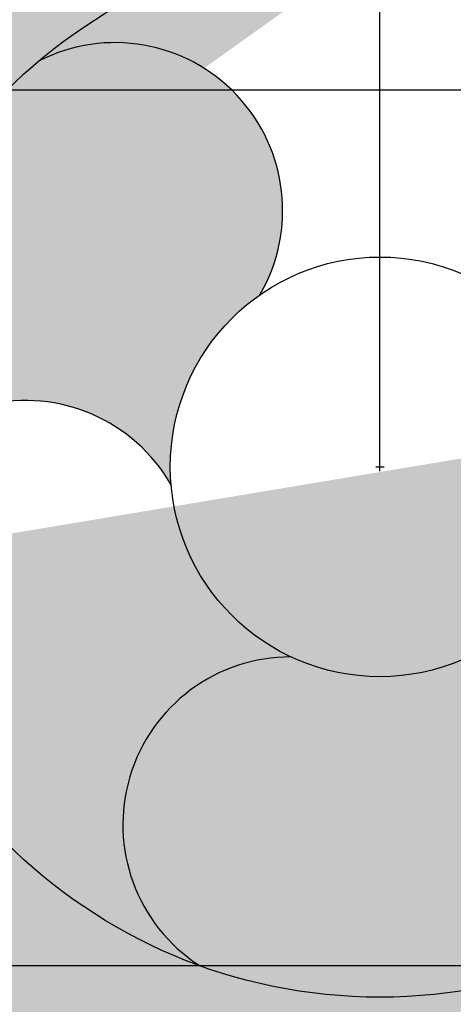
# Model space of a CAD drawing. Units: millimetres. Extents: x -22994 to 29398, y -19990 to 20176.
# Tile 116 of 135: x 220 to 229, y 135 to 156. Entities that reach past the tile are written whole.
import ezdxf

# ---------------------------------------------------------------- set-up
doc = ezdxf.new("R2010")
doc.units = ezdxf.units.MM
doc.header["$MEASUREMENT"] = 0
for name, color, linetype, lineweight in [('M-DIMS', 2, 'Continuous', 18), ('M-EQPM', 7, 'Continuous', 25), ('M-EQPM-PATT', 7, 'Continuous', 18)]:
    doc.layers.add(name, color=color, linetype=linetype, lineweight=lineweight)
doc.styles.get("Standard").update_dxf_attribs({"font": 'arial.ttf'})
doc.dimstyles.get("Standard").update_dxf_attribs({"dimtxt": 0.18, "dimasz": 10000, "dimexe": 0.18, "dimexo": 0.0625, "dimgap": 0.09, "dimtad": 0, "dimtih": 1, "dimtoh": 1, "dimdec": 0, "dimzin": 0, "dimdsep": 46, "dimtxsty": 'Standard', "dimcen": 0.09, "dimadec": 0, "dimazin": 0, "dimtfac": 1, "dimtdec": 0, "dimtofl": 0, "dimtmove": 0, "dimatfit": 3, "dimfxl": 1, "dimtolj": 1, "dimtzin": 0, "dimlwd": 30, "dimarcsym": 0})

# ---------------------------------------------------------------- blocks, each defined once
blk = doc.blocks.new('*D2')
at = {"layer": 'Defpoints', "color": 0, "transparency": 16777216}
for p in [(6.677, 10.271), (290.852, 10.271), (290.852, -5.079)]:
    blk.add_point(p, dxfattribs=at)
at = {"layer": 'M-DIMS', "color": 0, "lineweight": -2, "transparency": 16777216}
for p, q in [((6.677, 10.209), (6.677, -5.259)), ((290.852, 10.209), (290.852, -5.259))]:
    blk.add_line(p, q, dxfattribs=at)
at = {"layer": 'M-DIMS', "color": 0, "lineweight": 30, "transparency": 16777216}
for p, q in [((-9993.323, -5.079), (-19993.323, -5.079)), ((10290.852, -5.079), (20290.852, -5.079))]:
    blk.add_line(p, q, dxfattribs=at)
at = {"layer": 'M-DIMS', "color": 0, "transparency": 16777216}
for points in [[(-9993.323, 1661.588), (-9993.323, -1671.745), (6.677, -5.079)], [(10290.852, 1661.588), (10290.852, -1671.745), (290.852, -5.079)]]:
    blk.add_solid(points, dxfattribs=at)
at = {"layer": 'M-DIMS', "color": 0, "transparency": 16777216, "insert": (148.765, -5.079), "char_height": 0.18, "attachment_point": 5}
blk.add_mtext('\\A1;284.2', dxfattribs=at)
blk = doc.blocks.new('*D3')
at = {"layer": 'Defpoints', "color": 0, "transparency": 16777216}
for p in [(110.265, 204.165), (110.265, 176.366), (95.833, 127.967)]:
    blk.add_point(p, dxfattribs=at)
at = {"layer": 'M-DIMS', "color": 0, "lineweight": -2, "transparency": 16777216}
for p, q in [((95.833, 128.03), (95.833, 204.345)), ((110.265, 176.429), (110.265, 204.345))]:
    blk.add_line(p, q, dxfattribs=at)
at = {"layer": 'M-DIMS', "color": 0, "lineweight": 30, "transparency": 16777216}
for p, q in [((-9904.167, 204.165), (-19904.167, 204.165)), ((10110.265, 204.165), (20110.265, 204.165))]:
    blk.add_line(p, q, dxfattribs=at)
at = {"layer": 'M-DIMS', "color": 0, "transparency": 16777216}
for points in [[(-9904.167, 1870.832), (-9904.167, -1462.501), (95.833, 204.165)], [(10110.265, 1870.832), (10110.265, -1462.501), (110.265, 204.165)]]:
    blk.add_solid(points, dxfattribs=at)
at = {"layer": 'M-DIMS', "color": 0, "transparency": 16777216, "insert": (103.049, 204.165), "char_height": 0.18, "attachment_point": 5}
blk.add_mtext('\\A1;14.432', dxfattribs=at)
blk = doc.blocks.new('*D4')
at = {"layer": 'Defpoints', "color": 0, "transparency": 16777216}
for p in [(116.265, 204.165), (110.265, 176.366), (116.265, 176.366)]:
    blk.add_point(p, dxfattribs=at)
at = {"layer": 'M-DIMS', "color": 0, "lineweight": -2, "transparency": 16777216}
for p, q in [((110.265, 176.429), (110.265, 204.345)), ((116.265, 176.429), (116.265, 204.345))]:
    blk.add_line(p, q, dxfattribs=at)
at = {"layer": 'M-DIMS', "color": 0, "lineweight": 30, "transparency": 16777216}
for p, q in [((-9889.735, 204.165), (-19889.735, 204.165)), ((10116.265, 204.165), (20116.265, 204.165))]:
    blk.add_line(p, q, dxfattribs=at)
at = {"layer": 'M-DIMS', "color": 0, "transparency": 16777216}
for points in [[(-9889.735, 1870.832), (-9889.735, -1462.501), (110.265, 204.165)], [(10116.265, 1870.832), (10116.265, -1462.501), (116.265, 204.165)]]:
    blk.add_solid(points, dxfattribs=at)
at = {"layer": 'M-DIMS', "color": 0, "transparency": 16777216, "insert": (113.265, 204.165), "char_height": 0.18, "attachment_point": 5}
blk.add_mtext('\\A1;6', dxfattribs=at)
blk = doc.blocks.new('*D5')
at = {"layer": 'Defpoints', "color": 0, "transparency": 16777216}
for p in [(181.265, 204.165), (116.265, 176.366), (181.265, 176.366)]:
    blk.add_point(p, dxfattribs=at)
at = {"layer": 'M-DIMS', "color": 0, "lineweight": -2, "transparency": 16777216}
for p, q in [((116.265, 176.429), (116.265, 204.345)), ((181.265, 176.429), (181.265, 204.345))]:
    blk.add_line(p, q, dxfattribs=at)
at = {"layer": 'M-DIMS', "color": 0, "lineweight": 30, "transparency": 16777216}
for p, q in [((-9883.735, 204.165), (-19883.735, 204.165)), ((10181.265, 204.165), (20181.265, 204.165))]:
    blk.add_line(p, q, dxfattribs=at)
at = {"layer": 'M-DIMS', "color": 0, "transparency": 16777216}
for points in [[(-9883.735, 1870.832), (-9883.735, -1462.501), (116.265, 204.165)], [(10181.265, 1870.832), (10181.265, -1462.501), (181.265, 204.165)]]:
    blk.add_solid(points, dxfattribs=at)
at = {"layer": 'M-DIMS', "color": 0, "transparency": 16777216, "insert": (148.765, 204.165), "char_height": 0.18, "attachment_point": 5}
blk.add_mtext('\\A1;65', dxfattribs=at)
blk = doc.blocks.new('*D6')
at = {"layer": 'Defpoints', "color": 0, "transparency": 16777216}
for p in [(187.265, 204.165), (181.265, 176.366), (187.265, 176.366)]:
    blk.add_point(p, dxfattribs=at)
at = {"layer": 'M-DIMS', "color": 0, "lineweight": -2, "transparency": 16777216}
for p, q in [((181.265, 176.429), (181.265, 204.345)), ((187.265, 176.429), (187.265, 204.345))]:
    blk.add_line(p, q, dxfattribs=at)
at = {"layer": 'M-DIMS', "color": 0, "lineweight": 30, "transparency": 16777216}
for p, q in [((-9818.735, 204.165), (-19818.735, 204.165)), ((10187.265, 204.165), (20187.265, 204.165))]:
    blk.add_line(p, q, dxfattribs=at)
at = {"layer": 'M-DIMS', "color": 0, "transparency": 16777216}
for points in [[(-9818.735, 1870.832), (-9818.735, -1462.501), (181.265, 204.165)], [(10187.265, 1870.832), (10187.265, -1462.501), (187.265, 204.165)]]:
    blk.add_solid(points, dxfattribs=at)
at = {"layer": 'M-DIMS', "color": 0, "transparency": 16777216, "insert": (184.265, 204.165), "char_height": 0.18, "attachment_point": 5}
blk.add_mtext('\\A1;6', dxfattribs=at)
blk = doc.blocks.new('*D7')
at = {"layer": 'Defpoints', "color": 0, "transparency": 16777216}
for p in [(201.697, 204.165), (187.265, 176.366), (201.697, 127.967)]:
    blk.add_point(p, dxfattribs=at)
at = {"layer": 'M-DIMS', "color": 0, "lineweight": -2, "transparency": 16777216}
for p, q in [((187.265, 176.429), (187.265, 204.345)), ((201.697, 128.03), (201.697, 204.345))]:
    blk.add_line(p, q, dxfattribs=at)
at = {"layer": 'M-DIMS', "color": 0, "lineweight": 30, "transparency": 16777216}
for p, q in [((-9812.735, 204.165), (-19812.735, 204.165)), ((10201.697, 204.165), (20201.697, 204.165))]:
    blk.add_line(p, q, dxfattribs=at)
at = {"layer": 'M-DIMS', "color": 0, "transparency": 16777216}
for points in [[(-9812.735, 1870.832), (-9812.735, -1462.501), (187.265, 204.165)], [(10201.697, 1870.832), (10201.697, -1462.501), (201.697, 204.165)]]:
    blk.add_solid(points, dxfattribs=at)
at = {"layer": 'M-DIMS', "color": 0, "transparency": 16777216, "insert": (194.481, 204.165), "char_height": 0.18, "attachment_point": 5}
blk.add_mtext('\\A1;14.432', dxfattribs=at)
blk = doc.blocks.new('*D8')
at = {"layer": 'Defpoints', "color": 0, "transparency": 16777216}
for p in [(227.648, 204.165), (227.648, 146.73), (201.697, 127.967)]:
    blk.add_point(p, dxfattribs=at)
at = {"layer": 'M-DIMS', "color": 0, "lineweight": -2, "transparency": 16777216}
for p, q in [((201.697, 128.03), (201.697, 204.345)), ((227.648, 146.792), (227.648, 204.345))]:
    blk.add_line(p, q, dxfattribs=at)
at = {"layer": 'M-DIMS', "color": 0, "lineweight": 30, "transparency": 16777216}
for p, q in [((-9798.303, 204.165), (-19798.303, 204.165)), ((10227.648, 204.165), (20227.648, 204.165))]:
    blk.add_line(p, q, dxfattribs=at)
at = {"layer": 'M-DIMS', "color": 0, "transparency": 16777216}
for points in [[(-9798.303, 1870.832), (-9798.303, -1462.501), (201.697, 204.165)], [(10227.648, 1870.832), (10227.648, -1462.501), (227.648, 204.165)]]:
    blk.add_solid(points, dxfattribs=at)
at = {"layer": 'M-DIMS', "color": 0, "transparency": 16777216, "insert": (214.673, 204.165), "char_height": 0.18, "attachment_point": 5}
blk.add_mtext('\\A1;25.95', dxfattribs=at)
blk = doc.blocks.new('*D9')
at = {"layer": 'Defpoints', "color": 0, "transparency": 16777216}
for p in [(187.265, 176.366), (306.202, 176.366), (290.852, 10.271)]:
    blk.add_point(p, dxfattribs=at)
at = {"layer": 'M-DIMS', "color": 0, "lineweight": 30, "transparency": 16777216}
for p, q in [((306.202, 10176.366), (306.202, 20176.366)), ((306.202, -9989.729), (306.202, -19989.729))]:
    blk.add_line(p, q, dxfattribs=at)
at = {"layer": 'M-DIMS', "color": 0, "lineweight": -2, "transparency": 16777216}
for p, q in [((187.327, 176.366), (306.382, 176.366)), ((290.915, 10.271), (306.382, 10.271))]:
    blk.add_line(p, q, dxfattribs=at)
at = {"layer": 'M-DIMS', "color": 0, "transparency": 16777216}
for points in [[(-1360.465, 10176.366), (1972.869, 10176.366), (306.202, 176.366)], [(-1360.465, -9989.729), (1972.869, -9989.729), (306.202, 10.271)]]:
    blk.add_solid(points, dxfattribs=at)
at = {"layer": 'M-DIMS', "color": 0, "transparency": 16777216, "insert": (306.202, 93.319), "char_height": 0.18, "attachment_point": 5}
blk.add_mtext('\\A1;166.1', dxfattribs=at)
blk = doc.blocks.new('*D10')
at = {"layer": 'Defpoints', "color": 0, "transparency": 16777216}
for p in [(125.65, 136.071), (133.346, 136.071), (133.346, -5.079)]:
    blk.add_point(p, dxfattribs=at)
at = {"layer": 'M-DIMS', "color": 0, "lineweight": -2, "transparency": 16777216}
for p, q in [((125.65, 136.009), (125.65, -5.259)), ((133.346, 136.009), (133.346, -5.259))]:
    blk.add_line(p, q, dxfattribs=at)
at = {"layer": 'M-DIMS', "color": 0, "lineweight": 30, "transparency": 16777216}
for p, q in [((-9874.35, -5.079), (-19874.35, -5.079)), ((10133.346, -5.079), (20133.346, -5.079))]:
    blk.add_line(p, q, dxfattribs=at)
at = {"layer": 'M-DIMS', "color": 0, "transparency": 16777216}
for points in [[(-9874.35, 1661.588), (-9874.35, -1671.745), (125.65, -5.079)], [(10133.346, 1661.588), (10133.346, -1671.745), (133.346, -5.079)]]:
    blk.add_solid(points, dxfattribs=at)
at = {"layer": 'M-DIMS', "color": 0, "transparency": 16777216, "insert": (129.498, -5.079), "char_height": 0.18, "attachment_point": 5}
blk.add_mtext('\\A1;7.696', dxfattribs=at)
blk = doc.blocks.new('*D11')
at = {"layer": 'Defpoints', "color": 0, "transparency": 16777216}
for p in [(133.346, 136.071), (135.65, 136.071), (135.65, -5.079)]:
    blk.add_point(p, dxfattribs=at)
at = {"layer": 'M-DIMS', "color": 0, "lineweight": -2, "transparency": 16777216}
for p, q in [((133.346, 136.009), (133.346, -5.259)), ((135.65, 136.009), (135.65, -5.259))]:
    blk.add_line(p, q, dxfattribs=at)
at = {"layer": 'M-DIMS', "color": 0, "lineweight": 30, "transparency": 16777216}
for p, q in [((-9866.654, -5.079), (-19866.654, -5.079)), ((10135.65, -5.079), (20135.65, -5.079))]:
    blk.add_line(p, q, dxfattribs=at)
at = {"layer": 'M-DIMS', "color": 0, "transparency": 16777216}
for points in [[(-9866.654, 1661.588), (-9866.654, -1671.745), (133.346, -5.079)], [(10135.65, 1661.588), (10135.65, -1671.745), (135.65, -5.079)]]:
    blk.add_solid(points, dxfattribs=at)
at = {"layer": 'M-DIMS', "color": 0, "transparency": 16777216, "insert": (134.498, -5.079), "char_height": 0.18, "attachment_point": 5}
blk.add_mtext('\\A1;2.304', dxfattribs=at)
blk = doc.blocks.new('*D12')
at = {"layer": 'Defpoints', "color": 0, "transparency": 16777216}
for p in [(135.65, 136.071), (145.65, 136.071), (145.65, -5.079)]:
    blk.add_point(p, dxfattribs=at)
at = {"layer": 'M-DIMS', "color": 0, "lineweight": -2, "transparency": 16777216}
for p, q in [((135.65, 136.009), (135.65, -5.259)), ((145.65, 136.009), (145.65, -5.259))]:
    blk.add_line(p, q, dxfattribs=at)
at = {"layer": 'M-DIMS', "color": 0, "lineweight": 30, "transparency": 16777216}
for p, q in [((-9864.35, -5.079), (-19864.35, -5.079)), ((10145.65, -5.079), (20145.65, -5.079))]:
    blk.add_line(p, q, dxfattribs=at)
at = {"layer": 'M-DIMS', "color": 0, "transparency": 16777216}
for points in [[(-9864.35, 1661.588), (-9864.35, -1671.745), (135.65, -5.079)], [(10145.65, 1661.588), (10145.65, -1671.745), (145.65, -5.079)]]:
    blk.add_solid(points, dxfattribs=at)
at = {"layer": 'M-DIMS', "color": 0, "transparency": 16777216, "insert": (140.65, -5.079), "char_height": 0.18, "attachment_point": 5}
blk.add_mtext('\\A1;10', dxfattribs=at)
blk = doc.blocks.new('*D13')
at = {"layer": 'Defpoints', "color": 0, "transparency": 16777216}
for p in [(145.65, 136.071), (155.65, 136.071), (155.65, -5.079)]:
    blk.add_point(p, dxfattribs=at)
at = {"layer": 'M-DIMS', "color": 0, "lineweight": -2, "transparency": 16777216}
for p, q in [((145.65, 136.009), (145.65, -5.259)), ((155.65, 136.009), (155.65, -5.259))]:
    blk.add_line(p, q, dxfattribs=at)
at = {"layer": 'M-DIMS', "color": 0, "lineweight": 30, "transparency": 16777216}
for p, q in [((-9854.35, -5.079), (-19854.35, -5.079)), ((10155.65, -5.079), (20155.65, -5.079))]:
    blk.add_line(p, q, dxfattribs=at)
at = {"layer": 'M-DIMS', "color": 0, "transparency": 16777216}
for points in [[(-9854.35, 1661.588), (-9854.35, -1671.745), (145.65, -5.079)], [(10155.65, 1661.588), (10155.65, -1671.745), (155.65, -5.079)]]:
    blk.add_solid(points, dxfattribs=at)
at = {"layer": 'M-DIMS', "color": 0, "transparency": 16777216, "insert": (150.65, -5.079), "char_height": 0.18, "attachment_point": 5}
blk.add_mtext('\\A1;10', dxfattribs=at)
blk = doc.blocks.new('*D14')
at = {"layer": 'Defpoints', "color": 0, "transparency": 16777216}
for p in [(155.65, 136.071), (165.65, 136.071), (165.65, -5.079)]:
    blk.add_point(p, dxfattribs=at)
at = {"layer": 'M-DIMS', "color": 0, "lineweight": -2, "transparency": 16777216}
for p, q in [((155.65, 136.009), (155.65, -5.259)), ((165.65, 136.009), (165.65, -5.259))]:
    blk.add_line(p, q, dxfattribs=at)
at = {"layer": 'M-DIMS', "color": 0, "lineweight": 30, "transparency": 16777216}
for p, q in [((-9844.35, -5.079), (-19844.35, -5.079)), ((10165.65, -5.079), (20165.65, -5.079))]:
    blk.add_line(p, q, dxfattribs=at)
at = {"layer": 'M-DIMS', "color": 0, "transparency": 16777216}
for points in [[(-9844.35, 1661.588), (-9844.35, -1671.745), (155.65, -5.079)], [(10165.65, 1661.588), (10165.65, -1671.745), (165.65, -5.079)]]:
    blk.add_solid(points, dxfattribs=at)
at = {"layer": 'M-DIMS', "color": 0, "transparency": 16777216, "insert": (160.65, -5.079), "char_height": 0.18, "attachment_point": 5}
blk.add_mtext('\\A1;10', dxfattribs=at)
blk = doc.blocks.new('*D15')
at = {"layer": 'Defpoints', "color": 0, "transparency": 16777216}
for p in [(173.346, 154.788), (173.346, 136.071), (306.202, 136.071)]:
    blk.add_point(p, dxfattribs=at)
at = {"layer": 'M-DIMS', "color": 0, "lineweight": 30, "transparency": 16777216}
for p, q in [((306.202, 10154.788), (306.202, 20154.788)), ((306.202, -9863.929), (306.202, -19863.929))]:
    blk.add_line(p, q, dxfattribs=at)
at = {"layer": 'M-DIMS', "color": 0, "lineweight": -2, "transparency": 16777216}
for p, q in [((173.408, 154.788), (306.382, 154.788)), ((173.408, 136.071), (306.382, 136.071))]:
    blk.add_line(p, q, dxfattribs=at)
at = {"layer": 'M-DIMS', "color": 0, "transparency": 16777216}
for points in [[(-1360.465, 10154.788), (1972.869, 10154.788), (306.202, 154.788)], [(-1360.465, -9863.929), (1972.869, -9863.929), (306.202, 136.071)]]:
    blk.add_solid(points, dxfattribs=at)
at = {"layer": 'M-DIMS', "color": 0, "transparency": 16777216, "insert": (306.202, 145.43), "char_height": 0.18, "attachment_point": 5}
blk.add_mtext('\\A1;18.717', dxfattribs=at)
blk = doc.blocks.new('*D16')
at = {"layer": 'Defpoints', "color": 0, "transparency": 16777216}
for p in [(120.17, 204.165), (110.466, 48.035), (120.17, 48.035)]:
    blk.add_point(p, dxfattribs=at)
at = {"layer": 'M-DIMS', "color": 0, "lineweight": -2, "transparency": 16777216}
for p, q in [((110.466, 48.097), (110.466, 204.345)), ((120.17, 48.097), (120.17, 204.345))]:
    blk.add_line(p, q, dxfattribs=at)
at = {"layer": 'M-DIMS', "color": 0, "lineweight": 30, "transparency": 16777216}
for p, q in [((-9889.534, 204.165), (-19889.534, 204.165)), ((10120.17, 204.165), (20120.17, 204.165))]:
    blk.add_line(p, q, dxfattribs=at)
at = {"layer": 'M-DIMS', "color": 0, "transparency": 16777216}
for points in [[(-9889.534, 1870.832), (-9889.534, -1462.501), (110.466, 204.165)], [(10120.17, 1870.832), (10120.17, -1462.501), (120.17, 204.165)]]:
    blk.add_solid(points, dxfattribs=at)
at = {"layer": 'M-DIMS', "color": 0, "transparency": 16777216, "insert": (115.318, 204.165), "char_height": 0.18, "attachment_point": 5}
blk.add_mtext('\\A1;9.704', dxfattribs=at)
blk = doc.blocks.new('*D17')
at = {"layer": 'Defpoints', "color": 0, "transparency": 16777216}
for p in [(126.17, 204.165), (120.17, 48.035), (126.17, 48.035)]:
    blk.add_point(p, dxfattribs=at)
at = {"layer": 'M-DIMS', "color": 0, "lineweight": -2, "transparency": 16777216}
for p, q in [((120.17, 48.097), (120.17, 204.345)), ((126.17, 48.097), (126.17, 204.345))]:
    blk.add_line(p, q, dxfattribs=at)
at = {"layer": 'M-DIMS', "color": 0, "lineweight": 30, "transparency": 16777216}
for p, q in [((-9879.83, 204.165), (-19879.83, 204.165)), ((10126.17, 204.165), (20126.17, 204.165))]:
    blk.add_line(p, q, dxfattribs=at)
at = {"layer": 'M-DIMS', "color": 0, "transparency": 16777216}
for points in [[(-9879.83, 1870.832), (-9879.83, -1462.501), (120.17, 204.165)], [(10126.17, 1870.832), (10126.17, -1462.501), (126.17, 204.165)]]:
    blk.add_solid(points, dxfattribs=at)
at = {"layer": 'M-DIMS', "color": 0, "transparency": 16777216, "insert": (123.17, 204.165), "char_height": 0.18, "attachment_point": 5}
blk.add_mtext('\\A1;6', dxfattribs=at)
blk = doc.blocks.new('*D18')
at = {"layer": 'Defpoints', "color": 0, "transparency": 16777216}
for p in [(132.17, 204.165), (126.17, 48.035), (132.17, 48.035)]:
    blk.add_point(p, dxfattribs=at)
at = {"layer": 'M-DIMS', "color": 0, "lineweight": -2, "transparency": 16777216}
for p, q in [((126.17, 48.097), (126.17, 204.345)), ((132.17, 48.097), (132.17, 204.345))]:
    blk.add_line(p, q, dxfattribs=at)
at = {"layer": 'M-DIMS', "color": 0, "lineweight": 30, "transparency": 16777216}
for p, q in [((-9873.83, 204.165), (-19873.83, 204.165)), ((10132.17, 204.165), (20132.17, 204.165))]:
    blk.add_line(p, q, dxfattribs=at)
at = {"layer": 'M-DIMS', "color": 0, "transparency": 16777216}
for points in [[(-9873.83, 1870.832), (-9873.83, -1462.501), (126.17, 204.165)], [(10132.17, 1870.832), (10132.17, -1462.501), (132.17, 204.165)]]:
    blk.add_solid(points, dxfattribs=at)
at = {"layer": 'M-DIMS', "color": 0, "transparency": 16777216, "insert": (129.17, 204.165), "char_height": 0.18, "attachment_point": 5}
blk.add_mtext('\\A1;6', dxfattribs=at)
blk = doc.blocks.new('*D19')
at = {"layer": 'Defpoints', "color": 0, "transparency": 16777216}
for p in [(138.17, 204.165), (132.17, 48.035), (138.17, 48.035)]:
    blk.add_point(p, dxfattribs=at)
at = {"layer": 'M-DIMS', "color": 0, "lineweight": -2, "transparency": 16777216}
for p, q in [((132.17, 48.097), (132.17, 204.345)), ((138.17, 48.097), (138.17, 204.345))]:
    blk.add_line(p, q, dxfattribs=at)
at = {"layer": 'M-DIMS', "color": 0, "lineweight": 30, "transparency": 16777216}
for p, q in [((-9867.83, 204.165), (-19867.83, 204.165)), ((10138.17, 204.165), (20138.17, 204.165))]:
    blk.add_line(p, q, dxfattribs=at)
at = {"layer": 'M-DIMS', "color": 0, "transparency": 16777216}
for points in [[(-9867.83, 1870.832), (-9867.83, -1462.501), (132.17, 204.165)], [(10138.17, 1870.832), (10138.17, -1462.501), (138.17, 204.165)]]:
    blk.add_solid(points, dxfattribs=at)
at = {"layer": 'M-DIMS', "color": 0, "transparency": 16777216, "insert": (135.17, 204.165), "char_height": 0.18, "attachment_point": 5}
blk.add_mtext('\\A1;6', dxfattribs=at)
blk = doc.blocks.new('*D20')
at = {"layer": 'Defpoints', "color": 0, "transparency": 16777216}
for p in [(144.17, 204.165), (138.17, 48.035), (144.17, 48.035)]:
    blk.add_point(p, dxfattribs=at)
at = {"layer": 'M-DIMS', "color": 0, "lineweight": -2, "transparency": 16777216}
for p, q in [((138.17, 48.097), (138.17, 204.345)), ((144.17, 48.097), (144.17, 204.345))]:
    blk.add_line(p, q, dxfattribs=at)
at = {"layer": 'M-DIMS', "color": 0, "lineweight": 30, "transparency": 16777216}
for p, q in [((-9861.83, 204.165), (-19861.83, 204.165)), ((10144.17, 204.165), (20144.17, 204.165))]:
    blk.add_line(p, q, dxfattribs=at)
at = {"layer": 'M-DIMS', "color": 0, "transparency": 16777216}
for points in [[(-9861.83, 1870.832), (-9861.83, -1462.501), (138.17, 204.165)], [(10144.17, 1870.832), (10144.17, -1462.501), (144.17, 204.165)]]:
    blk.add_solid(points, dxfattribs=at)
at = {"layer": 'M-DIMS', "color": 0, "transparency": 16777216, "insert": (141.17, 204.165), "char_height": 0.18, "attachment_point": 5}
blk.add_mtext('\\A1;6', dxfattribs=at)
blk = doc.blocks.new('*D21')
at = {"layer": 'Defpoints', "color": 0, "transparency": 16777216}
for p in [(149.116, 204.165), (144.17, 48.035), (149.116, 48.035)]:
    blk.add_point(p, dxfattribs=at)
at = {"layer": 'M-DIMS', "color": 0, "lineweight": -2, "transparency": 16777216}
for p, q in [((144.17, 48.097), (144.17, 204.345)), ((149.116, 48.097), (149.116, 204.345))]:
    blk.add_line(p, q, dxfattribs=at)
at = {"layer": 'M-DIMS', "color": 0, "lineweight": 30, "transparency": 16777216}
for p, q in [((-9855.83, 204.165), (-19855.83, 204.165)), ((10149.116, 204.165), (20149.116, 204.165))]:
    blk.add_line(p, q, dxfattribs=at)
at = {"layer": 'M-DIMS', "color": 0, "transparency": 16777216}
for points in [[(-9855.83, 1870.832), (-9855.83, -1462.501), (144.17, 204.165)], [(10149.116, 1870.832), (10149.116, -1462.501), (149.116, 204.165)]]:
    blk.add_solid(points, dxfattribs=at)
at = {"layer": 'M-DIMS', "color": 0, "transparency": 16777216, "insert": (146.643, 204.165), "char_height": 0.18, "attachment_point": 5}
blk.add_mtext('\\A1;4.945', dxfattribs=at)
blk = doc.blocks.new('*D22')
at = {"layer": 'Defpoints', "color": 0, "transparency": 16777216}
for p in [(149.116, 30.99), (155.116, 30.99), (155.116, -5.079)]:
    blk.add_point(p, dxfattribs=at)
at = {"layer": 'M-DIMS', "color": 0, "lineweight": -2, "transparency": 16777216}
for p, q in [((149.116, 30.927), (149.116, -5.259)), ((155.116, 30.927), (155.116, -5.259))]:
    blk.add_line(p, q, dxfattribs=at)
at = {"layer": 'M-DIMS', "color": 0, "lineweight": 30, "transparency": 16777216}
for p, q in [((-9850.884, -5.079), (-19850.884, -5.079)), ((10155.116, -5.079), (20155.116, -5.079))]:
    blk.add_line(p, q, dxfattribs=at)
at = {"layer": 'M-DIMS', "color": 0, "transparency": 16777216}
for points in [[(-9850.884, 1661.588), (-9850.884, -1671.745), (149.116, -5.079)], [(10155.116, 1661.588), (10155.116, -1671.745), (155.116, -5.079)]]:
    blk.add_solid(points, dxfattribs=at)
at = {"layer": 'M-DIMS', "color": 0, "transparency": 16777216, "insert": (152.116, -5.079), "char_height": 0.18, "attachment_point": 5}
blk.add_mtext('\\A1;6', dxfattribs=at)
blk = doc.blocks.new('*D23')
at = {"layer": 'Defpoints', "color": 0, "transparency": 16777216}
for p in [(155.116, 30.99), (161.116, 30.99), (161.116, -5.079)]:
    blk.add_point(p, dxfattribs=at)
at = {"layer": 'M-DIMS', "color": 0, "lineweight": -2, "transparency": 16777216}
for p, q in [((155.116, 30.927), (155.116, -5.259)), ((161.116, 30.927), (161.116, -5.259))]:
    blk.add_line(p, q, dxfattribs=at)
at = {"layer": 'M-DIMS', "color": 0, "lineweight": 30, "transparency": 16777216}
for p, q in [((-9844.884, -5.079), (-19844.884, -5.079)), ((10161.116, -5.079), (20161.116, -5.079))]:
    blk.add_line(p, q, dxfattribs=at)
at = {"layer": 'M-DIMS', "color": 0, "transparency": 16777216}
for points in [[(-9844.884, 1661.588), (-9844.884, -1671.745), (155.116, -5.079)], [(10161.116, 1661.588), (10161.116, -1671.745), (161.116, -5.079)]]:
    blk.add_solid(points, dxfattribs=at)
at = {"layer": 'M-DIMS', "color": 0, "transparency": 16777216, "insert": (158.116, -5.079), "char_height": 0.18, "attachment_point": 5}
blk.add_mtext('\\A1;6', dxfattribs=at)
blk = doc.blocks.new('*D24')
at = {"layer": 'Defpoints', "color": 0, "transparency": 16777216}
for p in [(161.116, 30.99), (166.439, 30.99), (166.439, -5.079)]:
    blk.add_point(p, dxfattribs=at)
at = {"layer": 'M-DIMS', "color": 0, "lineweight": -2, "transparency": 16777216}
for p, q in [((161.116, 30.927), (161.116, -5.259)), ((166.439, 30.927), (166.439, -5.259))]:
    blk.add_line(p, q, dxfattribs=at)
at = {"layer": 'M-DIMS', "color": 0, "lineweight": 30, "transparency": 16777216}
for p, q in [((-9838.884, -5.079), (-19838.884, -5.079)), ((10166.439, -5.079), (20166.439, -5.079))]:
    blk.add_line(p, q, dxfattribs=at)
at = {"layer": 'M-DIMS', "color": 0, "transparency": 16777216}
for points in [[(-9838.884, 1661.588), (-9838.884, -1671.745), (161.116, -5.079)], [(10166.439, 1661.588), (10166.439, -1671.745), (166.439, -5.079)]]:
    blk.add_solid(points, dxfattribs=at)
at = {"layer": 'M-DIMS', "color": 0, "transparency": 16777216, "insert": (163.777, -5.079), "char_height": 0.18, "attachment_point": 5}
blk.add_mtext('\\A1;5.323', dxfattribs=at)
blk = doc.blocks.new('*D25')
at = {"layer": 'Defpoints', "color": 0, "transparency": 16777216}
for p in [(166.439, 30.99), (172.439, 30.99), (172.439, -5.079)]:
    blk.add_point(p, dxfattribs=at)
at = {"layer": 'M-DIMS', "color": 0, "lineweight": -2, "transparency": 16777216}
for p, q in [((166.439, 30.927), (166.439, -5.259)), ((172.439, 30.927), (172.439, -5.259))]:
    blk.add_line(p, q, dxfattribs=at)
at = {"layer": 'M-DIMS', "color": 0, "lineweight": 30, "transparency": 16777216}
for p, q in [((-9833.561, -5.079), (-19833.561, -5.079)), ((10172.439, -5.079), (20172.439, -5.079))]:
    blk.add_line(p, q, dxfattribs=at)
at = {"layer": 'M-DIMS', "color": 0, "transparency": 16777216}
for points in [[(-9833.561, 1661.588), (-9833.561, -1671.745), (166.439, -5.079)], [(10172.439, 1661.588), (10172.439, -1671.745), (172.439, -5.079)]]:
    blk.add_solid(points, dxfattribs=at)
at = {"layer": 'M-DIMS', "color": 0, "transparency": 16777216, "insert": (169.439, -5.079), "char_height": 0.18, "attachment_point": 5}
blk.add_mtext('\\A1;6', dxfattribs=at)
blk = doc.blocks.new('*D26')
at = {"layer": 'Defpoints', "color": 0, "transparency": 16777216}
for p in [(172.439, 30.99), (178.439, 30.99), (178.439, -5.079)]:
    blk.add_point(p, dxfattribs=at)
at = {"layer": 'M-DIMS', "color": 0, "lineweight": -2, "transparency": 16777216}
for p, q in [((172.439, 30.927), (172.439, -5.259)), ((178.439, 30.927), (178.439, -5.259))]:
    blk.add_line(p, q, dxfattribs=at)
at = {"layer": 'M-DIMS', "color": 0, "lineweight": 30, "transparency": 16777216}
for p, q in [((-9827.561, -5.079), (-19827.561, -5.079)), ((10178.439, -5.079), (20178.439, -5.079))]:
    blk.add_line(p, q, dxfattribs=at)
at = {"layer": 'M-DIMS', "color": 0, "transparency": 16777216}
for points in [[(-9827.561, 1661.588), (-9827.561, -1671.745), (172.439, -5.079)], [(10178.439, 1661.588), (10178.439, -1671.745), (178.439, -5.079)]]:
    blk.add_solid(points, dxfattribs=at)
at = {"layer": 'M-DIMS', "color": 0, "transparency": 16777216, "insert": (175.439, -5.079), "char_height": 0.18, "attachment_point": 5}
blk.add_mtext('\\A1;6', dxfattribs=at)
blk = doc.blocks.new('*D27')
at = {"layer": 'Defpoints', "color": 0, "transparency": 16777216}
for p in [(178.439, 30.99), (188.117, 30.99), (188.117, -5.079)]:
    blk.add_point(p, dxfattribs=at)
at = {"layer": 'M-DIMS', "color": 0, "lineweight": -2, "transparency": 16777216}
for p, q in [((178.439, 30.927), (178.439, -5.259)), ((188.117, 30.927), (188.117, -5.259))]:
    blk.add_line(p, q, dxfattribs=at)
at = {"layer": 'M-DIMS', "color": 0, "lineweight": 30, "transparency": 16777216}
for p, q in [((-9821.561, -5.079), (-19821.561, -5.079)), ((10188.117, -5.079), (20188.117, -5.079))]:
    blk.add_line(p, q, dxfattribs=at)
at = {"layer": 'M-DIMS', "color": 0, "transparency": 16777216}
for points in [[(-9821.561, 1661.588), (-9821.561, -1671.745), (178.439, -5.079)], [(10188.117, 1661.588), (10188.117, -1671.745), (188.117, -5.079)]]:
    blk.add_solid(points, dxfattribs=at)
at = {"layer": 'M-DIMS', "color": 0, "transparency": 16777216, "insert": (183.278, -5.079), "char_height": 0.18, "attachment_point": 5}
blk.add_mtext('\\A1;9.679', dxfattribs=at)
blk = doc.blocks.new('*D28')
at = {"layer": 'Defpoints', "color": 0, "transparency": 16777216}
for p in [(188.117, 48.035), (306.202, 48.035), (188.117, 30.99)]:
    blk.add_point(p, dxfattribs=at)
at = {"layer": 'M-DIMS', "color": 0, "lineweight": 30, "transparency": 16777216}
for p, q in [((306.202, 10048.035), (306.202, 20048.035)), ((306.202, -9969.01), (306.202, -19969.01))]:
    blk.add_line(p, q, dxfattribs=at)
at = {"layer": 'M-DIMS', "color": 0, "lineweight": -2, "transparency": 16777216}
for p, q in [((188.18, 48.035), (306.382, 48.035)), ((188.18, 30.99), (306.382, 30.99))]:
    blk.add_line(p, q, dxfattribs=at)
at = {"layer": 'M-DIMS', "color": 0, "transparency": 16777216}
for points in [[(-1360.465, 10048.035), (1972.869, 10048.035), (306.202, 48.035)], [(-1360.465, -9969.01), (1972.869, -9969.01), (306.202, 30.99)]]:
    blk.add_solid(points, dxfattribs=at)
at = {"layer": 'M-DIMS', "color": 0, "transparency": 16777216, "insert": (306.202, 39.512), "char_height": 0.18, "attachment_point": 5}
blk.add_mtext('\\A1;17.045', dxfattribs=at)
blk = doc.blocks.new('*D29')
at = {"layer": 'Defpoints', "color": 0, "transparency": 16777216}
for p in [(36.801, 80.045), (64.03, 80.045)]:
    blk.add_point(p, dxfattribs=at)
at = {"layer": 'M-DIMS', "color": 0, "lineweight": -2, "transparency": 16777216}
for p, q in [((50.325, 80.045), (50.505, 80.045)), ((50.415, 79.955), (50.415, 80.135))]:
    blk.add_line(p, q, dxfattribs=at)
at = {"layer": 'M-DIMS', "color": 0, "lineweight": 30, "transparency": 16777216}
blk.add_line((20064.03, 80.03), (10064.03, 80.038), dxfattribs=at)
at = {"layer": 'M-DIMS', "color": 0, "transparency": 16777216}
blk.add_solid([(10064.031, 1746.704), (10064.028, -1586.629), (64.03, 80.045)], dxfattribs=at)
at = {"layer": 'M-DIMS', "color": 0, "transparency": 16777216, "insert": (20064.521, 80.03), "char_height": 0.18, "attachment_point": 5}
blk.add_mtext('\\A1;∅27.23', dxfattribs=at)
blk = doc.blocks.new('*D30')
at = {"layer": 'Defpoints', "color": 0, "transparency": 16777216}
for p in [(216.315, 146.729), (238.982, 146.73)]:
    blk.add_point(p, dxfattribs=at)
at = {"layer": 'M-DIMS', "color": 0, "lineweight": 30, "transparency": 16777216}
blk.add_line((20238.982, 147.496), (10238.982, 147.113), dxfattribs=at)
at = {"layer": 'M-DIMS', "color": 0, "lineweight": -2, "transparency": 16777216}
for p, q in [((227.558, 146.73), (227.738, 146.73)), ((227.648, 146.64), (227.648, 146.82))]:
    blk.add_line(p, q, dxfattribs=at)
at = {"layer": 'M-DIMS', "color": 0, "transparency": 16777216}
blk.add_solid([(10238.918, 1813.78), (10239.046, -1519.554), (238.982, 146.73)], dxfattribs=at)
at = {"layer": 'M-DIMS', "color": 0, "transparency": 16777216, "insert": (20239.544, 147.496), "char_height": 0.18, "attachment_point": 5}
blk.add_mtext('\\A1;∅22.667', dxfattribs=at)
blk = doc.blocks.new('*D31')
at = {"layer": 'Defpoints', "color": 0, "transparency": 16777216}
for p in [(223.164, 146.729), (232.133, 146.73)]:
    blk.add_point(p, dxfattribs=at)
at = {"layer": 'M-DIMS', "color": 0, "lineweight": 30, "transparency": 16777216}
blk.add_line((20232.133, 148.666), (10232.133, 147.698), dxfattribs=at)
at = {"layer": 'M-DIMS', "color": 0, "lineweight": -2, "transparency": 16777216}
for p, q in [((227.558, 146.73), (227.738, 146.73)), ((227.648, 146.64), (227.648, 146.82))]:
    blk.add_line(p, q, dxfattribs=at)
at = {"layer": 'M-DIMS', "color": 0, "transparency": 16777216}
blk.add_solid([(10231.971, 1814.364), (10232.294, -1518.969), (232.133, 146.73)], dxfattribs=at)
at = {"layer": 'M-DIMS', "color": 0, "transparency": 16777216, "insert": (20232.625, 148.666), "char_height": 0.18, "attachment_point": 5}
blk.add_mtext('\\A1;∅8.969', dxfattribs=at)
blk = doc.blocks.new('*D34')
at = {"layer": 'Defpoints', "color": 0, "transparency": 16777216}
for p in [(178.58, 122.895), (176.812, 121.128)]:
    blk.add_point(p, dxfattribs=at)
at = {"layer": 'M-DIMS', "color": 0, "lineweight": 30, "transparency": 16777216}
for p, q in [((14322.436, 14263.311), (7250.508, 7193.103)), ((24322.436, 14263.311), (14322.436, 14263.311))]:
    blk.add_line(p, q, dxfattribs=at)
at = {"layer": 'M-DIMS', "color": 0, "lineweight": -2, "transparency": 16777216}
for p, q in [((176.812, 121.038), (176.812, 121.218)), ((176.722, 121.128), (176.902, 121.128))]:
    blk.add_line(p, q, dxfattribs=at)
at = {"layer": 'M-DIMS', "color": 0, "transparency": 16777216}
blk.add_solid([(6072.14, 8371.758), (8428.876, 6014.448), (178.58, 122.895)], dxfattribs=at)
at = {"layer": 'M-DIMS', "color": 0, "transparency": 16777216, "insert": (24322.97, 14263.311), "char_height": 0.18, "attachment_point": 5}
blk.add_mtext('\\A1;6X R2.5', dxfattribs=at)
blk = doc.blocks.new('*D36')
at = {"layer": 'Defpoints', "color": 0, "transparency": 16777216}
for p in [(46.39, 31.303), (46.387, 26.593)]:
    blk.add_point(p, dxfattribs=at)
at = {"layer": 'M-DIMS', "color": 0, "lineweight": 30, "transparency": 16777216}
for p, q in [((57.15, 20031.301), (51.77, 10031.302)), ((10057.15, 20031.301), (57.15, 20031.301))]:
    blk.add_line(p, q, dxfattribs=at)
at = {"layer": 'M-DIMS', "color": 0, "lineweight": -2, "transparency": 16777216}
for p, q in [((46.389, 28.858), (46.389, 29.038)), ((46.299, 28.948), (46.479, 28.948))]:
    blk.add_line(p, q, dxfattribs=at)
at = {"layer": 'M-DIMS', "color": 0, "transparency": 16777216}
blk.add_solid([(-1614.896, 10032.199), (1718.436, 10030.405), (46.39, 31.303)], dxfattribs=at)
at = {"layer": 'M-DIMS', "color": 0, "transparency": 16777216, "insert": (10057.554, 20031.301), "char_height": 0.18, "attachment_point": 5}
blk.add_mtext('\\A1;∅4.71', dxfattribs=at)
blk = doc.blocks.new('*D37')
at = {"layer": 'Defpoints', "color": 0, "transparency": 16777216}
for p in [(54.834, 118.615), (59.494, 118.614)]:
    blk.add_point(p, dxfattribs=at)
at = {"layer": 'M-DIMS', "color": 0, "lineweight": -2, "transparency": 16777216}
for p, q in [((57.164, 118.524), (57.164, 118.704)), ((57.074, 118.614), (57.254, 118.614))]:
    blk.add_line(p, q, dxfattribs=at)
at = {"layer": 'M-DIMS', "color": 0, "lineweight": 30, "transparency": 16777216}
blk.add_line((20059.493, 116.253), (10059.494, 117.434), dxfattribs=at)
at = {"layer": 'M-DIMS', "color": 0, "transparency": 16777216}
blk.add_solid([(10059.69, 1784.1), (10059.297, -1549.233), (59.494, 118.614)], dxfattribs=at)
at = {"layer": 'M-DIMS', "color": 0, "transparency": 16777216, "insert": (20059.985, 116.253), "char_height": 0.18, "attachment_point": 5}
blk.add_mtext('\\A1;∅4.659', dxfattribs=at)

msp = doc.modelspace()

# ---------------------------------------------------------------- hatches: boundary and pattern name
at = {"layer": 'M-EQPM-PATT'}
h = msp.add_hatch(color=256, dxfattribs=at)
h.set_gradient(color1=(0, 0, 255), color2=(244, 238, 81), tint=1, name='CYLINDER')
h.paths.add_polyline_path([(232.1163, 147.1148, 0.7475711), (238.8087, 148.7044, 0.2679492), (231.5183, 157.3821, -0.7475711), (229.5488, 150.7914, -0.2679492)])
h.paths.add_polyline_path([(216.3148, 146.7296, 0.0438131), (216.4882, 144.7547, -0.7475711), (223.1807, 146.3444, -0.0215046), (223.1641, 146.7296, -0.2450326), (225.081, 150.4062, 0.7475711), (220.3581, 155.4072, 0.2215353)])
h.paths.add_polyline_path([(234.9389, 138.0519, -0.7475711), (230.216, 143.053, -0.2679492), (225.7482, 142.6678, 0.7475711), (223.7786, 136.0771, 0.2679492)])

# ---------------------------------------------------------------- linework, layer by layer
at = {"layer": 'M-EQPM'}
for radius in [11.3336, 4.4843]:
    msp.add_circle((227.6485, 146.7296), radius, dxfattribs=at)
for centre, start, end in [((221.9818, 152.2099), 329.80022, 116.92313), ((220.069, 144.5622), 29.80022, 176.92313), ((225.7357, 139.0819), 89.80022, 236.92313)]:
    msp.add_arc(centre, 3.5859, start, end, dxfattribs=at)

# ---------------------------------------------------------------- dimensions: what is measured, and where the dimension line sits
at = {"layer": 'M-DIMS'}
for base, p1, p2, override, picture, middle in [((306.202, 176.3662), (290.852, 10.2713), (187.2647, 176.3662), {"dimdec": 1, "dimlfac": 1, "dimrnd": 0, "dimzin": 0, "dimdsep": 46, "dimlunit": 2}, '*D9', (306.202, 93.3187)), ((306.202, 136.0713), (173.3459, 154.788), (173.3459, 136.0713), {"dimdec": 3, "dimlfac": 1, "dimrnd": 0, "dimzin": 0, "dimdsep": 46, "dimlunit": 2}, '*D15', (306.202, 145.4297)), ((306.202, 48.0349), (188.1175, 30.9895), (188.1175, 48.0349), {"dimdec": 3, "dimlfac": 1, "dimrnd": 0, "dimzin": 0, "dimdsep": 46, "dimlunit": 2}, '*D28', (306.202, 39.5122))]:
    dim = msp.add_linear_dim(base=base, p1=p1, p2=p2, angle=90, dimstyle='Standard', override=override, dxfattribs=at)
    dim.commit()
    dim.dimension.update_dxf_attribs({"geometry": picture, "text_midpoint": middle})
for p1, p2, override, picture, middle in [((46.3875, 26.5934), (46.39, 31.3035), {"dimdec": 2, "dimlfac": 1, "dimrnd": 0, "dimzin": 0, "dimdsep": 46, "dimlunit": 2}, '*D36', (10057.5542, 20031.3006)), ((223.1641, 146.7291), (232.1328, 146.73), {"dimdec": 3, "dimlfac": 1, "dimrnd": 0, "dimzin": 0, "dimdsep": 46, "dimlunit": 2}, '*D31', (20232.1327, 148.6656)), ((216.3148, 146.7291), (238.9821, 146.73), {"dimdec": 3, "dimlfac": 1, "dimrnd": 0, "dimzin": 0, "dimdsep": 46, "dimlunit": 2}, '*D30', (20238.9821, 147.4959))]:
    dim = msp.add_diameter_dim_2p(p1=p1, p2=p2, dimstyle='Standard', override=override, dxfattribs=at)
    dim.commit()
    dim.dimension.update_dxf_attribs({"geometry": picture, "text_midpoint": middle, "dimtype": 163})
dim = msp.add_radius_dim(center=(176.8123, 121.1277), mpoint=(178.5802, 122.8952), text='6X <>', dimstyle='Standard', override={"dimdec": 1, "dimlfac": 1, "dimrnd": 0, "dimzin": 0, "dimdsep": 46, "dimlunit": 2}, dxfattribs=at)
dim.commit()
dim.dimension.update_dxf_attribs({"geometry": '*D34', "text_midpoint": (24322.9703, 14263.3108)})
for base, p1, p2, override, picture, middle in [((110.2647, 204.1654), (95.8327, 127.967), (110.2647, 176.3662), {"dimdec": 3, "dimlfac": 1, "dimrnd": 0, "dimzin": 0, "dimdsep": 46, "dimlunit": 2}, '*D3', (103.0487, 204.1654)), ((116.2647, 204.1654), (110.2647, 176.3662), (116.2647, 176.3662), {"dimdec": 0, "dimlfac": 1, "dimrnd": 0, "dimzin": 0, "dimdsep": 46, "dimlunit": 2}, '*D4', (113.2647, 204.1654)), ((120.1702, 204.1654), (110.4658, 48.0349), (120.1702, 48.0349), {"dimdec": 3, "dimlfac": 1, "dimrnd": 0, "dimzin": 0, "dimdsep": 46, "dimlunit": 2}, '*D16', (115.318, 204.1654)), ((181.2647, 204.1654), (116.2647, 176.3662), (181.2647, 176.3662), {"dimdec": 0, "dimlfac": 1, "dimrnd": 0, "dimzin": 0, "dimdsep": 46, "dimlunit": 2}, '*D5', (148.7647, 204.1654)), ((126.1702, 204.1654), (120.1702, 48.0349), (126.1702, 48.0349), {"dimdec": 0, "dimlfac": 1, "dimrnd": 0, "dimzin": 0, "dimdsep": 46, "dimlunit": 2}, '*D17', (123.1702, 204.1654)), ((132.1702, 204.1654), (126.1702, 48.0349), (132.1702, 48.0349), {"dimdec": 0, "dimlfac": 1, "dimrnd": 0, "dimzin": 0, "dimdsep": 46, "dimlunit": 2}, '*D18', (129.1702, 204.1654)), ((138.1702, 204.1654), (132.1702, 48.0349), (138.1702, 48.0349), {"dimdec": 0, "dimlfac": 1, "dimrnd": 0, "dimzin": 0, "dimdsep": 46, "dimlunit": 2}, '*D19', (135.1702, 204.1654)), ((144.1702, 204.1654), (138.1702, 48.0349), (144.1702, 48.0349), {"dimdec": 0, "dimlfac": 1, "dimrnd": 0, "dimzin": 0, "dimdsep": 46, "dimlunit": 2}, '*D20', (141.1702, 204.1654)), ((149.11567, 204.16539), (144.17023, 48.03494), (149.11567, 48.03494), {"dimdec": 3, "dimlfac": 1, "dimrnd": 0, "dimzin": 0, "dimdsep": 46, "dimlunit": 2}, '*D21', (146.64295, 204.16539)), ((187.2647, 204.1654), (181.2647, 176.3662), (187.2647, 176.3662), {"dimdec": 0, "dimlfac": 1, "dimrnd": 0, "dimzin": 0, "dimdsep": 46, "dimlunit": 2}, '*D6', (184.2647, 204.1654)), ((201.6967, 204.1654), (187.2647, 176.3662), (201.6967, 127.967), {"dimdec": 3, "dimlfac": 1, "dimrnd": 0, "dimzin": 0, "dimdsep": 46, "dimlunit": 2}, '*D7', (194.4807, 204.1654)), ((227.6485, 204.1654), (201.6967, 127.967), (227.6485, 146.7296), {"dimdec": 2, "dimlfac": 1, "dimrnd": 0, "dimzin": 0, "dimdsep": 46, "dimlunit": 2}, '*D8', (214.6726, 204.1654)), ((290.852, -5.0787), (6.6773, 10.2713), (290.852, 10.2713), {"dimdec": 1, "dimlfac": 1, "dimrnd": 0, "dimzin": 0, "dimdsep": 46, "dimlunit": 2}, '*D2', (148.7647, -5.0787)), ((133.3459, -5.0787), (125.6498, 136.0713), (133.3459, 136.0713), {"dimdec": 3, "dimlfac": 1, "dimrnd": 0, "dimzin": 0, "dimdsep": 46, "dimlunit": 2}, '*D10', (129.4978, -5.0787)), ((135.6498, -5.0787), (133.3459, 136.0713), (135.6498, 136.0713), {"dimdec": 3, "dimlfac": 1, "dimrnd": 0, "dimzin": 0, "dimdsep": 46, "dimlunit": 2}, '*D11', (134.4978, -5.0787)), ((145.6498, -5.0787), (135.6498, 136.0713), (145.6498, 136.0713), {"dimdec": 0, "dimlfac": 1, "dimrnd": 0, "dimzin": 0, "dimdsep": 46, "dimlunit": 2}, '*D12', (140.6498, -5.0787)), ((155.6498, -5.0787), (145.6498, 136.0713), (155.6498, 136.0713), {"dimdec": 0, "dimlfac": 1, "dimrnd": 0, "dimzin": 0, "dimdsep": 46, "dimlunit": 2}, '*D13', (150.6498, -5.0787)), ((155.1157, -5.0787), (149.1157, 30.9895), (155.1157, 30.9895), {"dimdec": 0, "dimlfac": 1, "dimrnd": 0, "dimzin": 0, "dimdsep": 46, "dimlunit": 2}, '*D22', (152.1157, -5.0787)), ((161.1157, -5.0787), (155.1157, 30.9895), (161.1157, 30.9895), {"dimdec": 0, "dimlfac": 1, "dimrnd": 0, "dimzin": 0, "dimdsep": 46, "dimlunit": 2}, '*D23', (158.1157, -5.0787)), ((165.6498, -5.0787), (155.6498, 136.0713), (165.6498, 136.0713), {"dimdec": 0, "dimlfac": 1, "dimrnd": 0, "dimzin": 0, "dimdsep": 46, "dimlunit": 2}, '*D14', (160.6498, -5.0787)), ((166.4387, -5.0787), (161.1157, 30.9895), (166.4387, 30.9895), {"dimdec": 3, "dimlfac": 1, "dimrnd": 0, "dimzin": 0, "dimdsep": 46, "dimlunit": 2}, '*D24', (163.7772, -5.0787)), ((172.4387, -5.0787), (166.4387, 30.9895), (172.4387, 30.9895), {"dimdec": 0, "dimlfac": 1, "dimrnd": 0, "dimzin": 0, "dimdsep": 46, "dimlunit": 2}, '*D25', (169.4387, -5.0787)), ((178.4387, -5.0787), (172.4387, 30.9895), (178.4387, 30.9895), {"dimdec": 0, "dimlfac": 1, "dimrnd": 0, "dimzin": 0, "dimdsep": 46, "dimlunit": 2}, '*D26', (175.4387, -5.0787)), ((188.1175, -5.0787), (178.4387, 30.9895), (188.1175, 30.9895), {"dimdec": 3, "dimlfac": 1, "dimrnd": 0, "dimzin": 0, "dimdsep": 46, "dimlunit": 2}, '*D27', (183.2781, -5.0787))]:
    dim = msp.add_linear_dim(base=base, p1=p1, p2=p2, dimstyle='Standard', override=override, dxfattribs=at)
    dim.commit()
    dim.dimension.update_dxf_attribs({"geometry": picture, "text_midpoint": middle})
for p1, p2, override, picture, middle in [((54.8343, 118.6145), (59.4936, 118.614), {"dimdec": 3, "dimlfac": 1, "dimrnd": 0, "dimzin": 0, "dimdsep": 46, "dimlunit": 2}, '*D37', (20059.4934, 116.2531)), ((36.8006, 80.045), (64.0296, 80.045), {"dimdec": 2, "dimlfac": 1, "dimrnd": 0, "dimzin": 0, "dimdsep": 46, "dimlunit": 2}, '*D29', (20064.0296, 80.0303))]:
    dim = msp.add_diameter_dim_2p(p1=p1, p2=p2, dimstyle='Standard', override=override, dxfattribs=at)
    dim.commit()
    dim.dimension.update_dxf_attribs({"geometry": picture, "text_midpoint": middle})

doc.saveas('drawing.dxf')
